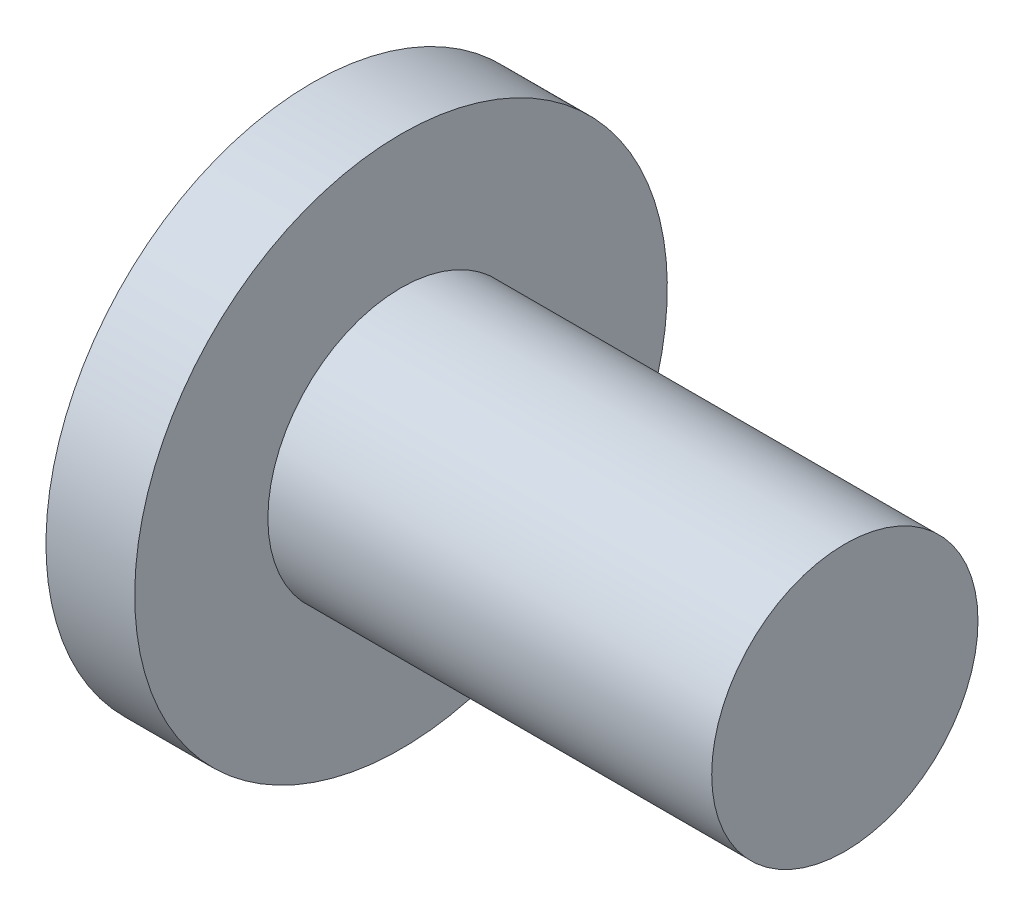
from build123d import *


with BuildPart() as part:
    # Pin Profile Sketch → Headed Pin Revolve (revolve)
    with BuildSketch(Plane.XY):
        Polygon((0, 0), (-12, 0), (-12, 6), (-10, 6), (-10, 3), (0, 3), align=None)
    revolve(axis=Axis((0, 0, 0), (-1, 0, 0)))


solid = part.part
